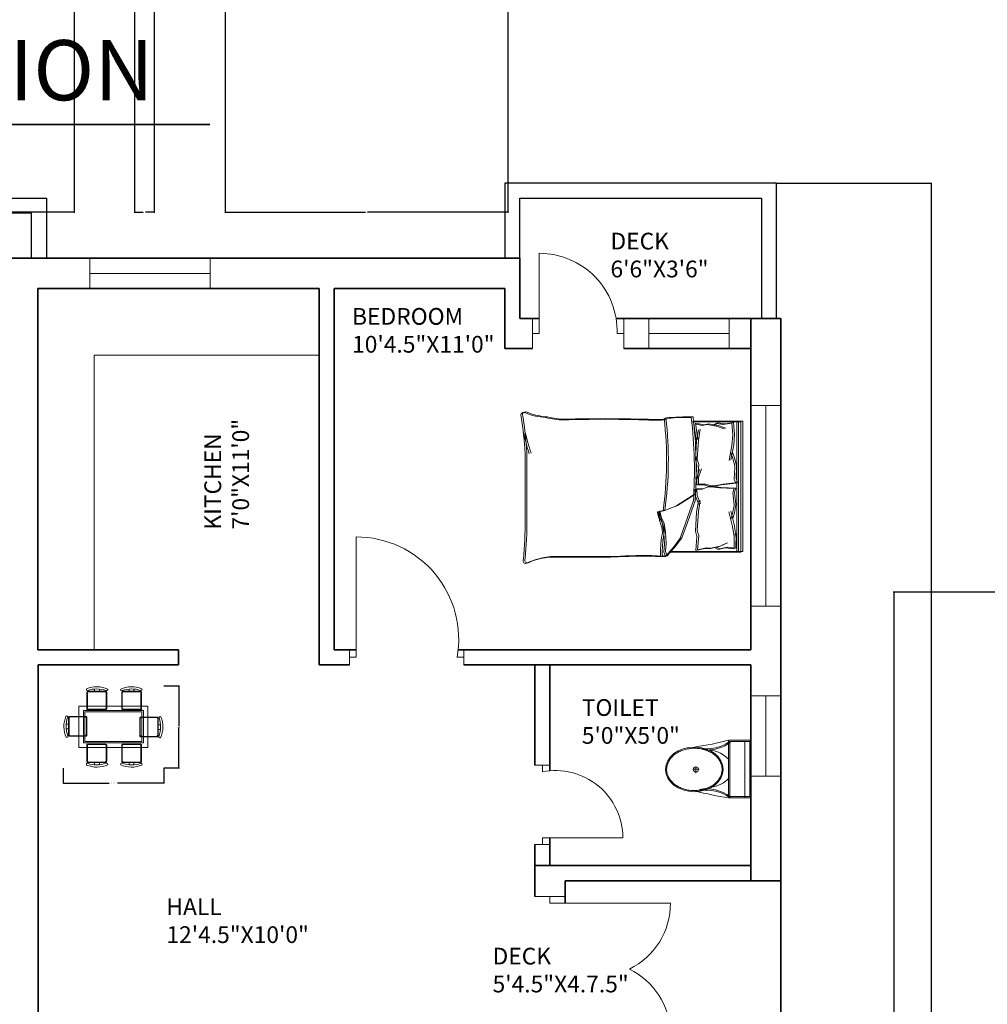
# Model space of a CAD drawing. Units: inches. Extents: x 2250 to 3629, y 982 to 2740.
# Tile 5 of 12: x 2629 to 2918, y 1825 to 2119. Entities that reach past the tile are written whole.
import ezdxf

# ---------------------------------------------------------------- set-up
doc = ezdxf.new("R2010")
doc.units = ezdxf.units.IN
for name, color, linetype, lineweight in [('A-ANNO-DIMS', 2, 'Continuous', 18), ('A-ANNO-TITL', 7, 'Continuous', 35), ('A-AREA-IDEN', 7, 'Continuous', 18), ('A-DOOR', 3, 'Continuous', 18), ('A-FLOR-DECK', 7, 'Continuous', 25), ('A-FLOR-FIXT', 9, 'Continuous', 18), ('A-FURN', 8, 'Continuous', 13), ('A-GLAZ', 4, 'Continuous', 18), ('A-WALL', 7, 'Continuous', 35)]:
    doc.layers.add(name, color=color, linetype=linetype, lineweight=lineweight)
doc.styles.get("Standard").update_dxf_attribs({"font": 'arial.ttf'})
doc.dimstyles.get("Standard").update_dxf_attribs({"dimtxt": 0.18, "dimasz": 0.18, "dimexe": 0.18, "dimexo": 0.0625, "dimgap": 0.09, "dimtad": 0, "dimtih": 1, "dimtoh": 1, "dimdec": 4, "dimzin": 0, "dimdsep": 46, "dimtxsty": 'Standard', "dimcen": 0.09, "dimadec": 0, "dimazin": 0, "dimtfac": 1, "dimtdec": 4, "dimtofl": 0, "dimtmove": 0, "dimatfit": 3, "dimfxl": 1, "dimtolj": 1, "dimtzin": 0, "dimarcsym": 0})

# ---------------------------------------------------------------- blocks, each defined once
blk = doc.blocks.new('A$C31115884')
for p, q in [((283.1, 497.7), (223.4, 497.7)), ((257.5, 466.4), (257.5, 523.2)), ((0, 200), (0, 0)), ((520, 200), (0, 200)), ((10, 190), (10, 10)), ((510, 190), (10, 190)), ((510, 10), (510, 190)), ((520, 0), (520, 200)), ((510, 54.5), (0, 54.5)), ((10, 10), (510, 10)), ((0, 0), (520, 0))]:
    blk.add_line(p, q)
blk.add_circle((255.6, 496.4), 23.6)
for centre, radius, start, end in [((2777.7, -204.6), 2807, 165.4549, 171.71327), ((-294.5, 403.3), 364.7, 324.20913, 9.34987), ((-294.5, 403.3), 374.7, 324.20913, 9.34987), ((805.8, 403.3), 364.7, 170.65013, 215.79087), ((3237, 905), 2807, 188.28673, 194.5451), ((139.5, 406.2), 293.5, 315.84364, 2.65635), ((805.8, 403.3), 374.7, 179.20365, 215.79087), ((383.6, 406.2), 293.5, 190.27735, 224.15636)]:
    blk.add_arc(centre, radius, start, end)
blk.add_ellipse((256.2, 509.9), major_axis=(0, -260.7), ratio=0.772727)
blk.add_open_spline([(256.2, 259.2), (263.1, 259.2), (270, 259.7), (287.8, 262.3), (298.7, 265.1), (319.9, 273.1), (330.2, 278.4), (350.1, 291.1), (359.7, 298.7), (377.7, 315.9), (386.2, 325.5), (401.7, 346.6), (408.8, 358.1), (421.3, 382.5), (426.8, 395.5), (435.9, 422.4), (439.5, 436.4), (444.8, 465.1), (446.5, 479.7), (447.9, 509.2), (447.6, 524), (445, 553.3), (442.7, 567.8), (436.3, 596), (432.1, 609.7), (421.9, 636), (416, 648.6), (402.5, 672.1), (395, 683), (378.6, 703), (369.8, 712.1), (351.1, 728), (341.3, 734.8), (320.9, 746.2), (310.4, 750.7), (288.9, 757.3), (278, 759.4), (256, 761), (245, 760.6), (223.1, 757.2), (212.3, 754.3), (191.1, 746.1), (180.8, 740.7), (160.9, 727.8), (151.4, 720.1), (133.5, 702.7), (125.1, 693), (109.6, 671.7), (102.6, 660.2), (90.2, 635.7), (84.9, 622.7), (76, 595.6), (72.4, 581.6), (67.2, 552.9), (65.6, 538.2), (64.4, 508.8), (64.8, 494), (67.5, 464.7), (69.9, 450.2), (76.6, 422), (80.8, 408.3), (91.1, 382.2), (97.2, 369.7), (110.8, 346.3), (118.4, 335.4), (134.8, 315.6), (143.7, 306.7), (162.4, 290.9), (172.3, 284.2), (192.8, 273), (203.3, 268.6), (224.8, 262.2), (235.8, 260.2), (249.9, 259.3), (253, 259.2), (256.2, 259.2)], degree=3, knots=[0, 0, 0, 0, 0.110105, 0.110105, 0.285049, 0.285049, 0.459994, 0.459994, 0.634938, 0.634938, 0.809882, 0.809882, 0.984827, 0.984827, 1.159771, 1.159771, 1.334715, 1.334715, 1.50966, 1.50966, 1.684604, 1.684604, 1.859549, 1.859549, 2.034493, 2.034493, 2.209437, 2.209437, 2.384382, 2.384382, 2.559326, 2.559326, 2.73427, 2.73427, 2.909215, 2.909215, 3.084159, 3.084159, 3.259103, 3.259103, 3.434048, 3.434048, 3.608992, 3.608992, 3.783936, 3.783936, 3.958881, 3.958881, 4.133825, 4.133825, 4.30877, 4.30877, 4.483714, 4.483714, 4.658658, 4.658658, 4.833603, 4.833603, 5.008547, 5.008547, 5.183491, 5.183491, 5.358436, 5.358436, 5.53338, 5.53338, 5.708324, 5.708324, 5.883269, 5.883269, 6.058213, 6.058213, 6.233158, 6.233158, 6.283185, 6.283185, 6.283185, 6.283185])
blk = doc.blocks.new('DR-36-BED-NE')
for p, q in [((2, 2.25), (2, 38.25)), ((0, 4.5), (0, 0)), ((34.14, 4.5), (34.14, 0)), ((0, 0), (0, 2.25)), ((0, 2.25), (2, 2.25)), ((34.14, 2.25), (32.14, 2.25)), ((34.14, 0), (34.14, 2.25))]:
    blk.add_line(p, q)
blk.add_arc((2, 7.63), 30.62, 349.8775, 90)
blk = doc.blocks.new('DR-24-DECK-NE')
for p, q in [((2, 4.5), (2, 28.5)), ((0, 9), (0, 0)), ((27.25, 9), (27.25, 0)), ((0, 0), (0, 4.5)), ((0, 4.5), (2, 4.5)), ((27.25, 4.5), (25.25, 4.5)), ((27.25, 0), (27.25, 4.5))]:
    blk.add_line(p, q)
blk.add_arc((2, 5.23), 23.27, 358.191, 90)
blk = doc.blocks.new('DR-24-BATH-NE')
for p, q in [((0, 23.65), (4.5, 23.65)), ((4.5, 23.65), (2.25, 23.65)), ((2.25, 23.65), (2.25, 21.65)), ((4.5, 0), (0, 0)), ((0, 0), (0, 0)), ((0, 0), (2.25, 0)), ((2.25, 0), (2.25, 2)), ((2.25, 2), (26.25, 2))]:
    blk.add_line(p, q)
blk.add_arc((6.2, 2), 20.05, 0, 101.3787)
blk = doc.blocks.new('DR-72-DECK-EAST-N')
for p, q in [((9, 42.6), (0, 42.6)), ((0, 42.6), (4.5, 42.6)), ((4.5, 42.6), (4.5, 40.6)), ((4.5, 40.6), (40.5, 40.6)), ((9, 0), (0, 0)), ((0, 0), (4.5, 0)), ((4.5, 0), (4.5, 2)), ((4.5, 2), (40.5, 2))]:
    blk.add_line(p, q)
for centre, radius, start, end in [((18.63, 40.6), 21.87, 295.9981, 0), ((18.59, 1.24), 21.93, 1.9829, 63.9515)]:
    blk.add_arc(centre, radius, start, end)
blk = doc.blocks.new('WIN-24-DECK-NE')
for p, q in [((0, 4.5), (0, 9)), ((0, 9), (0, 0)), ((24, 0), (24, 9)), ((24, 9), (24, 4.5)), ((24, 4.5), (0, 4.5))]:
    blk.add_line(p, q)
blk = doc.blocks.new('WIN-60-BED-NE')
for p, q in [((0, 60), (9, 60)), ((9, 60), (4.5, 60)), ((4.5, 60), (4.5, 12)), ((4.5, 12), (4.5, 0)), ((4.5, 0), (0, 0)), ((0, 0), (9, 0))]:
    blk.add_line(p, q)
blk = doc.blocks.new('WIN-36-KITCHEN-NE')
for p, q in [((0, 9), (0, 0)), ((0, 0), (0, 9)), ((0, 9), (0, 4.5)), ((36, 4.5), (36, 9)), ((36, 9), (36, 0)), ((0, 4.5), (36, 4.5))]:
    blk.add_line(p, q)
blk = doc.blocks.new('WIN-24-BATH-NW')
for p, q in [((9, 24), (0, 24)), ((0, 24), (4.5, 24)), ((4.5, 24), (4.5, 0)), ((9, 0), (0, 0)), ((4.5, 0), (9, 0))]:
    blk.add_line(p, q)
blk = doc.blocks.new('BED-WITH-PILLOWS')
for p, q in [((2.83, 51.56), (2.83, 66.3)), ((2.83, 66.3), (41.74, 66.3)), ((2.83, 65.05), (41.74, 65.05)), ((3.02, 51.04), (3.02, 65.78)), ((3.02, 65.78), (41.92, 65.78)), ((19.98, 64.31), (21.15, 64.78)), ((21.15, 64.78), (21.62, 60.43)), ((41.74, 66.3), (41.74, 44.64)), ((41.92, 65.78), (41.92, 44.12)), ((3.02, 64.53), (41.92, 64.53)), ((3.17, 63.59), (6.66, 63.85)), ((3.17, 63.6), (3.64, 61.01)), ((3.36, 63.06), (6.85, 63.33)), ((3.36, 63.08), (3.83, 60.49)), ((6.66, 63.85), (6.75, 63.84)), ((6.75, 63.84), (9.86, 63.6)), ((6.85, 63.33), (6.93, 63.32)), ((6.93, 63.32), (10.04, 63.08)), ((9.86, 63.6), (14.33, 62.78)), ((10.04, 63.08), (14.52, 62.26)), ((12.09, 63.25), (13.74, 63.84)), ((12.28, 62.73), (13.93, 63.32)), ((13.74, 63.84), (16.09, 64.43)), ((13.93, 63.32), (16.28, 63.91)), ((16.09, 64.43), (16.36, 64.43)), ((16.28, 63.91), (16.54, 63.91)), ((16.36, 64.43), (19.98, 64.31)), ((16.54, 63.91), (20.16, 63.79)), ((20.16, 63.79), (21.34, 64.26)), ((21.34, 64.26), (21.81, 59.9)), ((22.78, 64.27), (22.58, 59.9)), ((22.96, 63.75), (22.76, 59.38)), ((23.98, 63.88), (22.78, 64.27)), ((24.17, 63.36), (22.96, 63.75)), ((27.59, 64.22), (23.98, 63.88)), ((27.77, 63.7), (24.17, 63.36)), ((27.85, 64.24), (27.59, 64.22)), ((28.03, 63.72), (27.77, 63.7)), ((30.23, 63.8), (27.85, 64.24)), ((30.42, 63.28), (28.03, 63.72)), ((34.12, 63.8), (29.71, 62.7)), ((34.31, 63.28), (29.9, 62.18)), ((31.91, 63.31), (30.23, 63.8)), ((32.1, 62.79), (30.42, 63.28)), ((37.22, 64.23), (34.12, 63.8)), ((37.4, 63.71), (34.31, 63.28)), ((40.8, 64.22), (36.4, 64.3)), ((36.4, 64.3), (37.22, 64.23)), ((40.98, 63.7), (36.58, 63.78)), ((36.58, 63.78), (37.4, 63.71)), ((40.8, 64.22), (40.49, 61.61)), ((40.98, 63.7), (40.67, 61.09)), ((3.64, 61.01), (3.29, 58.89)), ((3.29, 58.89), (3.76, 58.07)), ((3.83, 60.49), (3.47, 58.37)), ((3.64, 56.07), (4.11, 59.01)), ((4.11, 59.01), (4.94, 61.25)), ((4.3, 58.49), (5.12, 60.73)), ((21.62, 60.43), (22.09, 57.84)), ((21.81, 59.9), (22.28, 57.32)), ((22.58, 59.9), (22.27, 57.28)), ((22.76, 59.38), (22.46, 56.76)), ((40.14, 59.58), (39.18, 61.76)), ((40.33, 59.06), (39.37, 61.24)), ((40.8, 56.67), (40.14, 59.58)), ((40.98, 56.15), (40.33, 59.06)), ((40.49, 61.61), (40.97, 59.51)), ((40.97, 59.51), (40.55, 58.66)), ((40.67, 61.09), (41.16, 58.99)), ((41.16, 58.99), (40.74, 58.14)), ((3.47, 58.37), (3.95, 57.55)), ((3.88, 54.78), (3.64, 56.07)), ((3.83, 55.55), (4.3, 58.49)), ((22.09, 56.78), (21.62, 55.25)), ((22.28, 56.26), (21.81, 54.73)), ((22.09, 57.84), (22.09, 56.78)), ((22.27, 57.28), (22.34, 56.23)), ((22.28, 57.32), (22.28, 56.26)), ((22.34, 56.23), (22.9, 54.73)), ((22.46, 56.76), (22.52, 55.71)), ((40.64, 55.37), (40.8, 56.67)), ((40.83, 54.85), (40.98, 56.15)), ((3.41, 52.19), (3.88, 54.78)), ((3.59, 51.66), (4.06, 54.25)), ((4.06, 54.25), (3.83, 55.55)), ((5.2, 53.58), (8.48, 53.04)), ((5.38, 53.06), (8.66, 52.52)), ((8.48, 53.04), (7.56, 52.77)), ((8.48, 53.04), (14.18, 52.69)), ((14.18, 52.69), (15.78, 53.14)), ((15.78, 53.14), (19.96, 52.81)), ((19.62, 53.06), (17.06, 53.95)), ((19.81, 52.54), (17.25, 53.43)), ((21.62, 53.06), (19.62, 53.06)), ((21.62, 55.25), (21.62, 53.06)), ((21.81, 54.73), (21.81, 52.54)), ((22.52, 55.71), (23.09, 54.21)), ((22.9, 54.73), (23.04, 52.55)), ((23.09, 54.21), (23.22, 52.03)), ((25.03, 52.68), (27.53, 53.72)), ((25.22, 52.15), (27.72, 53.2)), ((26.51, 53.58), (29.79, 53.04)), ((26.7, 53.06), (29.98, 52.52)), ((29.79, 53.04), (35.5, 52.69)), ((35.5, 52.69), (37.1, 53.14)), ((37.1, 53.14), (41.27, 52.81)), ((41.27, 52.81), (40.64, 55.37)), ((41.46, 52.29), (40.83, 54.85)), ((7.56, 52.77), (3.41, 52.19)), ((7.74, 52.25), (3.59, 51.66)), ((8.66, 52.52), (7.74, 52.25)), ((8.66, 52.52), (14.37, 52.17)), ((14.37, 52.17), (15.97, 52.62)), ((15.97, 52.62), (20.14, 52.29)), ((21.81, 52.54), (19.81, 52.54)), ((23.04, 52.55), (25.03, 52.68)), ((23.22, 52.03), (25.22, 52.15)), ((24.63, 52.15), (28.05, 46.86)), ((24.82, 51.63), (28.23, 46.34)), ((33.09, 49.76), (26.3, 52.15)), ((33.27, 49.24), (26.49, 51.63)), ((29.98, 52.52), (35.69, 52.17)), ((35.69, 52.17), (37.28, 52.62)), ((37.28, 52.62), (41.46, 52.29)), ((37.63, 48.12), (33.09, 49.76)), ((37.81, 47.6), (33.27, 49.24)), ((40.02, 46.36), (37.63, 48.12)), ((40.21, 45.84), (37.81, 47.6)), ((28.05, 46.86), (29.43, 43.21)), ((28.23, 46.34), (29.62, 42.69)), ((43.04, 43.71), (40.02, 46.36)), ((43.23, 43.19), (40.21, 45.84)), ((29.43, 43.21), (29.68, 41.57)), ((29.62, 42.69), (29.87, 41.05)), ((29.68, 41.57), (31.7, 42.08)), ((29.87, 41.05), (31.89, 41.56)), ((31.7, 42.08), (33.34, 42.83)), ((31.89, 41.56), (33.53, 42.31)), ((33.34, 42.83), (36.11, 43.21)), ((33.53, 42.31), (36.3, 42.69)), ((36.11, 43.21), (39.27, 43.46)), ((36.3, 42.69), (39.45, 42.94)), ((39.27, 43.46), (41.79, 43.21)), ((39.45, 42.94), (41.97, 42.69)), ((41.79, 43.21), (43.04, 43.71)), ((41.97, 42.69), (43.23, 43.19)), ((43.1, 42.29), (43.04, 43.71, 3.15)), ((43.29, 41.77), (43.23, 43.19, 3.15)), ((12.26, 1.79), (32.3, 1.79)), ((12.45, 1.27), (32.49, 1.27))]:
    blk.add_line(p, q)
for centre, radius, start, end in [((69.33, 49.94), 67.82, 178.7218, 185.604), ((17.39, -81.91), 134.3, 86.0865, 96.7821), ((69.52, 49.42), 67.82, 178.7218, 185.604), ((17.57, -82.43), 134.3, 86.0865, 96.7821), ((14.46, -60.96), 105.04, 81.7845, 96.9006), ((14.64, -61.48), 105.04, 81.7845, 96.9006), ((-136.21, 40.92), 138.49, 358.4762, 1.0082), ((-136.02, 40.4), 138.49, 358.4762, 1.0082), ((29.83, 41.52), 0.15, 160.2464, 271.1377), ((25.36, 65.1), 24.14, 280.6617, 289.8806), ((25.55, 64.58), 24.14, 280.6617, 289.8806), ((35.61, 37.76), 5.07, 78.6608, 113.7384), ((35.8, 37.23), 5.07, 78.6608, 113.7384), ((41.79, 71.72), 29.46, 259.8763, 272.5657), ((41.97, 71.2), 29.46, 259.8763, 272.5657), ((148.38, 36.74), 105.43, 176.9791, 183.8365), ((148.57, 36.22), 105.43, 176.9791, 183.8365), ((30.01, 41), 0.15, 160.2464, 271.1377), ((394.7, 25.1), 392.65, 178.2277, 181.7185), ((394.88, 24.58), 392.65, 178.2277, 181.7185), ((-3670.6, 11.09), 3713.84, 0.00217, 0.28689), ((-3670.41, 10.57), 3713.84, 0.00217, 0.28689), ((-21.9, 13.78), 24.13, 346.0648, 358.9113), ((-21.71, 13.26), 24.13, 346.0648, 358.9113), ((62, 10.4), 18.78, 177.4714, 206.4681), ((62.19, 9.88), 18.78, 177.4714, 206.4681), ((-17.63, 9.09), 19.18, 337.9751, 356.652), ((-17.45, 8.57), 19.18, 337.9751, 356.652), ((-14.02, 85.61), 86.67, 283.3832, 287.7053), ((0.89, 1.4), 0.887, 146.1736, 293.4781), ((1.07, 0.88), 0.887, 146.1736, 293.4781), ((17.44, -97.2), 99.12, 92.9958, 99.4091), ((17.63, -97.72), 99.12, 92.9958, 99.4091), ((-13.83, 85.09), 86.67, 283.3832, 287.7053), ((33.5, -106.51), 108.31, 84.4998, 90.6351), ((33.69, -107.03), 108.31, 84.4998, 90.6351), ((44.3, 2.09), 0.897, 242.6588, 356.02), ((44.48, 1.57), 0.897, 242.6588, 356.02)]:
    blk.add_arc(centre, radius, start, end)
blk = doc.blocks.new('DINING-SET-6')
for points in [[(7.06, 22.9, -0.175809), (12.68, 22.86, 0.578392), (13.1, 23.32, 0.214524), (6.77, 23.41, 0.552014), (7.06, 22.9, -0.065079)], [(17.4, 22.86, -0.578392), (16.98, 23.32, -0.214524), (23.31, 23.41, -0.552014), (23.02, 22.9, 0.175809), (17.4, 22.86)], [(12.44, 22.67), (7.23, 22.67, 0.414214), (6.86, 22.31), (6.86, 17.52, 0.414214), (7.23, 17.15), (12.44, 17.15, 0.414214), (12.8, 17.52), (12.8, 22.31, 0.414214), (12.44, 22.67)], [(10.61, 22.67), (10.61, 23.33, -0.064759)], [(22.85, 22.67, -0.414214), (23.22, 22.31), (23.22, 17.52, -0.414214), (22.85, 17.15), (17.64, 17.15, -0.414214), (17.28, 17.52), (17.28, 22.31, -0.414214), (17.64, 22.67), (22.85, 22.67)], [(19.47, 22.67), (19.47, 23.33, 0.064759)], [(1.19, 9.34, -0.578392), (0.72, 8.92, -0.214524), (0.64, 15.25, -0.552014), (1.15, 14.96, 0.175809), (1.19, 9.34)], [(1.37, 14.79, -0.414214), (1.74, 15.16), (6.53, 15.16, -0.414214), (6.89, 14.79), (6.89, 9.58, -0.414214), (6.53, 9.22), (1.74, 9.22, -0.414214), (1.37, 9.58), (1.37, 14.79)], [(28.21, 14.61, 0.414214), (27.85, 14.98), (23.05, 14.98, 0.414214), (22.69, 14.61), (22.69, 9.4, 0.414214), (23.05, 9.04), (27.85, 9.04, 0.414214), (28.21, 9.4), (28.21, 14.61)], [(28.44, 14.78, -0.175809), (28.39, 9.16, 0.578392), (28.86, 8.74, 0.214524), (28.95, 15.08, 0.552014), (28.44, 14.78, -0.065079)], [(1.37, 11.41), (0.71, 11.41, 0.064759)], [(28.21, 11.23), (28.87, 11.23, -0.064759)], [(12.44, 1.37), (7.23, 1.37, -0.414214), (6.86, 1.74), (6.86, 6.53, -0.414214), (7.23, 6.89), (12.44, 6.89, -0.414214), (12.8, 6.53), (12.8, 1.74, -0.414214), (12.44, 1.37)], [(22.85, 1.37, 0.414214), (23.22, 1.74), (23.22, 6.53, 0.414214), (22.85, 6.89), (17.64, 6.89, 0.414214), (17.28, 6.53), (17.28, 1.74, 0.414214), (17.64, 1.37), (22.85, 1.37)], [(12.68, 1.19, -0.578392), (13.1, 0.72, -0.214524), (6.77, 0.64, -0.552014), (7.06, 1.15, 0.175809), (12.68, 1.19)], [(10.61, 1.37), (10.61, 0.71, 0.064759)], [(23.02, 1.15, -0.175809), (17.4, 1.19, 0.578392), (16.98, 0.72, 0.214524), (23.31, 0.64, 0.552014), (23.02, 1.15, -0.065079)], [(19.47, 1.37), (19.47, 0.71, -0.064759)]]:
    blk.add_lwpolyline(points, format="xyb")
for points in [[(7.23, 22.51), (12.27, 22.51, -0.414214), (12.64, 22.15), (12.64, 17.68, -0.414214), (12.27, 17.32), (7.23, 17.32, -0.512069), (7.03, 17.68), (7.03, 22.15, -0.512069)], [(22.85, 22.51), (17.81, 22.51, 0.414214), (17.44, 22.15), (17.44, 17.68, 0.414214), (17.81, 17.32), (22.85, 17.32, 0.512069), (23.05, 17.68), (23.05, 22.15, 0.512069)], [(1.54, 14.79), (1.54, 9.75, 0.414214), (1.9, 9.38), (6.37, 9.38, 0.414214), (6.73, 9.75), (6.73, 14.79, 0.512069), (6.37, 14.99), (1.9, 14.99, 0.512069)], [(28.05, 14.61), (28.05, 9.57, -0.414214), (27.68, 9.2), (23.22, 9.2, -0.414214), (22.85, 9.57), (22.85, 14.61, -0.512069), (23.22, 14.81), (27.68, 14.81, -0.512069)], [(7.23, 1.54), (12.27, 1.54, 0.414214), (12.64, 1.9), (12.64, 6.36, 0.414214), (12.27, 6.73), (7.23, 6.73, 0.512069), (7.03, 6.36), (7.03, 1.9, 0.512069)], [(22.85, 1.54), (17.81, 1.54, -0.414214), (17.44, 1.9), (17.44, 6.36, -0.414214), (17.81, 6.73), (22.85, 6.73, -0.512069), (23.05, 6.36), (23.05, 1.9, -0.512069)]]:
    blk.add_lwpolyline(points, format="xyb", close=True)
for points in [[(9.15, 23.35), (9.15, 22.67)], [(20.93, 23.35), (20.93, 22.67)], [(0.7, 12.87), (1.37, 12.87)], [(28.88, 12.69), (28.21, 12.69)], [(9.15, 0.7), (9.15, 1.37)], [(20.93, 0.7), (20.93, 1.37)]]:
    blk.add_lwpolyline(points)
for points in [[(4.51, 18.27), (25.12, 18.27), (25.12, 5.91), (4.51, 5.91)], [(5.89, 16.9), (23.75, 16.9), (23.75, 7.28), (5.89, 7.28)], [(6.3, 16.49), (23.34, 16.49), (23.34, 7.69), (6.3, 7.69)]]:
    blk.add_lwpolyline(points, close=True)
blk = doc.blocks.new('*D61')
at = {"layer": 'A-ANNO-DIMS', "color": 0, "lineweight": -2, "transparency": 16777216}
for p, q in [((2642.11, 1895.36), (2642.11, 1890.73)), ((2672.18, 1895.36), (2672.18, 1890.73)), ((2642.29, 1890.91), (2655.86, 1890.91)), ((2672, 1890.91), (2658.42, 1890.91))]:
    blk.add_line(p, q, dxfattribs=at)
at = {"layer": 'A-ANNO-DIMS', "color": 0, "transparency": 16777216}
for points in [[(2642.29, 1890.94), (2642.29, 1890.88), (2642.11, 1890.91)], [(2672, 1890.94), (2672, 1890.88), (2672.18, 1890.91)]]:
    blk.add_solid(points, dxfattribs=at)
at = {"layer": 'Defpoints', "color": 0, "transparency": 16777216}
for p in [(2642.11, 1895.42), (2672.18, 1895.42), (2672.18, 1890.91)]:
    blk.add_point(p, dxfattribs=at)
at = {"layer": 'A-ANNO-DIMS', "color": 0, "transparency": 16777216, "insert": (2657.14, 1890.91), "char_height": 0.18, "attachment_point": 5}
blk.add_mtext('\\A1;DINING SET 30 TYP.', dxfattribs=at)
blk = doc.blocks.new('*D62')
at = {"layer": 'A-ANNO-DIMS', "color": 0, "lineweight": -2, "transparency": 16777216}
for p, q in [((2672.24, 1919.95), (2676.87, 1919.95)), ((2676.69, 1919.77), (2676.69, 1907.87)), ((2676.69, 1895.6), (2676.69, 1907.5)), ((2672.24, 1895.42), (2676.87, 1895.42))]:
    blk.add_line(p, q, dxfattribs=at)
at = {"layer": 'A-ANNO-DIMS', "color": 0, "transparency": 16777216}
for points in [[(2676.66, 1919.77), (2676.72, 1919.77), (2676.69, 1919.95)], [(2676.66, 1895.6), (2676.72, 1895.6), (2676.69, 1895.42)]]:
    blk.add_solid(points, dxfattribs=at)
at = {"layer": 'Defpoints', "color": 0, "transparency": 16777216}
for p in [(2672.18, 1919.95), (2676.69, 1919.95), (2672.18, 1895.42)]:
    blk.add_point(p, dxfattribs=at)
at = {"layer": 'A-ANNO-DIMS', "color": 0, "transparency": 16777216, "insert": (2676.69, 1907.69), "char_height": 0.18, "attachment_point": 5}
blk.add_mtext('\\A1;25 TYP.', dxfattribs=at)
blk = doc.blocks.new('*D170')
at = {"layer": 'A-ANNO-DIMS', "color": 0, "lineweight": -2, "transparency": 16777216}
for p, q in [((2855.4, 2070.24), (2901.69, 2070.24)), ((2901.51, 2070.06), (2901.51, 1664.67)), ((2901.51, 1258.92), (2901.51, 1664.3)), ((2481.67, 1258.74), (2901.69, 1258.74))]:
    blk.add_line(p, q, dxfattribs=at)
at = {"layer": 'A-ANNO-DIMS', "color": 0, "transparency": 16777216}
for points in [[(2901.48, 2070.06), (2901.54, 2070.06), (2901.51, 2070.24)], [(2901.48, 1258.92), (2901.54, 1258.92), (2901.51, 1258.74)]]:
    blk.add_solid(points, dxfattribs=at)
at = {"layer": 'Defpoints', "color": 0, "transparency": 16777216}
for p in [(2855.34, 2070.24), (2901.51, 2070.24), (2481.61, 1258.74)]:
    blk.add_point(p, dxfattribs=at)
at = {"layer": 'A-ANNO-DIMS', "color": 0, "transparency": 16777216, "insert": (2901.51, 1664.49), "char_height": 0.18, "attachment_point": 5}
blk.add_mtext('\\A1;811.5', dxfattribs=at)
blk = doc.blocks.new('*D173')
at = {"layer": 'A-ANNO-DIMS', "color": 0, "lineweight": -2, "transparency": 16777216}
for p, q in [((2932.01, 1947.92), (2890.14, 1947.92)), ((2890.32, 1947.74), (2890.32, 1603.51)), ((2890.32, 1258.92), (2890.32, 1603.15)), ((2981.16, 1258.74), (2890.14, 1258.74))]:
    blk.add_line(p, q, dxfattribs=at)
at = {"layer": 'A-ANNO-DIMS', "color": 0, "transparency": 16777216}
for points in [[(2890.29, 1947.74), (2890.35, 1947.74), (2890.32, 1947.92)], [(2890.29, 1258.92), (2890.35, 1258.92), (2890.32, 1258.74)]]:
    blk.add_solid(points, dxfattribs=at)
at = {"layer": 'Defpoints', "color": 0, "transparency": 16777216}
for p in [(2932.07, 1947.92), (2890.32, 1258.74), (2981.23, 1258.74)]:
    blk.add_point(p, dxfattribs=at)
at = {"layer": 'A-ANNO-DIMS', "color": 0, "transparency": 16777216, "insert": (2890.32, 1603.33), "char_height": 0.18, "attachment_point": 5}
blk.add_mtext('\\A1;689.2', dxfattribs=at)
blk = doc.blocks.new('*D184')
at = {"layer": 'A-ANNO-DIMS', "color": 0, "lineweight": -2, "transparency": 16777216}
for p, q in [((2645.41, 2191.68), (2645.41, 2061.34)), ((2597.69, 2173.64), (2597.69, 2061.34)), ((2597.87, 2061.52), (2621.08, 2061.52)), ((2645.23, 2061.52), (2622.02, 2061.52))]:
    blk.add_line(p, q, dxfattribs=at)
at = {"layer": 'A-ANNO-DIMS', "color": 0, "transparency": 16777216}
for points in [[(2597.87, 2061.55), (2597.87, 2061.49), (2597.69, 2061.52)], [(2645.23, 2061.55), (2645.23, 2061.49), (2645.41, 2061.52)]]:
    blk.add_solid(points, dxfattribs=at)
at = {"layer": 'Defpoints', "color": 0, "transparency": 16777216}
for p in [(2645.41, 2191.74), (2597.69, 2173.7), (2645.41, 2061.52)]:
    blk.add_point(p, dxfattribs=at)
at = {"layer": 'A-ANNO-DIMS', "color": 0, "transparency": 16777216, "insert": (2621.55, 2061.52), "char_height": 0.18, "attachment_point": 5}
blk.add_mtext('\\A1;47.725', dxfattribs=at)
blk = doc.blocks.new('*D185')
at = {"layer": 'A-ANNO-DIMS', "color": 0, "lineweight": -2, "transparency": 16777216}
for p, q in [((2663.46, 2191.6), (2663.46, 2061.34)), ((2669.31, 2191.64), (2669.31, 2061.34)), ((2663.64, 2061.52), (2666.06, 2061.52)), ((2669.13, 2061.52), (2666.71, 2061.52))]:
    blk.add_line(p, q, dxfattribs=at)
at = {"layer": 'A-ANNO-DIMS', "color": 0, "transparency": 16777216}
for points in [[(2663.64, 2061.55), (2663.64, 2061.49), (2663.46, 2061.52)], [(2669.13, 2061.55), (2669.13, 2061.49), (2669.31, 2061.52)]]:
    blk.add_solid(points, dxfattribs=at)
at = {"layer": 'Defpoints', "color": 0, "transparency": 16777216}
for p in [(2663.46, 2191.66), (2669.31, 2191.7), (2669.31, 2061.52)]:
    blk.add_point(p, dxfattribs=at)
at = {"layer": 'A-ANNO-DIMS', "color": 0, "transparency": 16777216, "insert": (2666.38, 2061.52), "char_height": 0.18, "attachment_point": 5}
blk.add_mtext('\\A1;5.85', dxfattribs=at)
blk = doc.blocks.new('*D186')
at = {"layer": 'A-ANNO-DIMS', "color": 0, "lineweight": -2, "transparency": 16777216}
for p, q in [((2690.54, 2191.64), (2690.54, 2061.34)), ((2775.05, 2173.64), (2775.05, 2061.34)), ((2690.72, 2061.52), (2732.47, 2061.52)), ((2774.87, 2061.52), (2733.12, 2061.52))]:
    blk.add_line(p, q, dxfattribs=at)
at = {"layer": 'A-ANNO-DIMS', "color": 0, "transparency": 16777216}
for points in [[(2690.72, 2061.55), (2690.72, 2061.49), (2690.54, 2061.52)], [(2774.87, 2061.55), (2774.87, 2061.49), (2775.05, 2061.52)]]:
    blk.add_solid(points, dxfattribs=at)
at = {"layer": 'Defpoints', "color": 0, "transparency": 16777216}
for p in [(2690.54, 2191.7), (2775.05, 2173.7), (2775.05, 2061.52)]:
    blk.add_point(p, dxfattribs=at)
at = {"layer": 'A-ANNO-DIMS', "color": 0, "transparency": 16777216, "insert": (2732.8, 2061.52), "char_height": 0.18, "attachment_point": 5}
blk.add_mtext('\\A1;84.5', dxfattribs=at)

msp = doc.modelspace()

# ---------------------------------------------------------------- linework, layer by layer
at = {"layer": 'A-ANNO-TITL'}
msp.add_line((2533.1975, 2087.7229), (2686.0181, 2087.7229), dxfattribs=at)
at = {"layer": 'A-FLOR-DECK'}
for p, q in [((2855.3384, 2070.2354), (2774.1072, 2070.2354)), ((2774.1072, 2070.2354), (2774.1072, 2047.7354)), ((2855.3384, 2065.7354), (2855.3384, 2070.2354)), ((2562.1345, 2065.7354), (2637.208, 2065.7354)), ((2637.208, 2065.7354), (2637.208, 2047.7354)), ((2778.6072, 2047.7354), (2778.6072, 2065.7354)), ((2778.6072, 2065.7354), (2850.8384, 2065.7354)), ((2850.8384, 2065.7354), (2850.8384, 2029.7354)), ((2855.3384, 2029.7354), (2855.3384, 2065.7354)), ((2632.708, 2061.2354), (2566.6345, 2061.2354)), ((2632.708, 2047.7354), (2632.708, 2061.2354)), ((2637.208, 2047.7354), (2632.708, 2047.7354))]:
    msp.add_line(p, q, dxfattribs=at)
at = {"layer": 'A-FLOR-FIXT'}
for p, q in [((2651.3954, 1930.7354), (2651.3954, 2018.7457)), ((2651.3954, 2018.7457), (2718.6072, 2018.7457))]:
    msp.add_line(p, q, dxfattribs=at)
at = {"layer": 'A-WALL'}
for p, q in [((2625.6072, 2047.7354), (2778.6072, 2047.7354)), ((2778.6072, 2047.7354), (2778.6072, 2029.7354)), ((2634.6072, 2038.7354), (2634.6072, 1930.7354)), ((2634.6072, 2038.7354), (2718.6072, 2038.7354)), ((2718.6072, 2038.7354), (2718.6072, 1930.7354)), ((2723.1072, 2038.7354), (2723.1072, 1930.7354)), ((2723.1072, 2038.7354), (2774.1072, 2038.7354)), ((2774.1072, 2020.7354), (2774.1072, 2038.7354)), ((2778.6072, 2029.7354), (2784.402, 2029.7354)), ((2807.3608, 2029.7354), (2847.6072, 2029.7354)), ((2847.6072, 2029.7354), (2847.6072, 1930.7354)), ((2847.6072, 2029.7354), (2847.6072, 2020.7354)), ((2847.6072, 2029.7354), (2856.6072, 2029.7354)), ((2856.6072, 2029.7354), (2856.6072, 1276.7354)), ((2778.6072, 2020.7354), (2774.1072, 2020.7354)), ((2782.402, 2020.7354), (2778.6072, 2020.7354)), ((2847.6072, 2020.7354), (2809.656, 2020.7354)), ((2634.6072, 1930.7354), (2676.6072, 1930.7354)), ((2676.6072, 1930.7354), (2676.6072, 1926.2354)), ((2718.6072, 1930.7354), (2718.6072, 1926.2354)), ((2723.1072, 1930.7354), (2729.7087, 1930.7354)), ((2760.1669, 1930.7354), (2847.6072, 1930.7354)), ((2634.7014, 1926.2354), (2634.7014, 1789.7354)), ((2634.7014, 1926.2354), (2676.6072, 1926.2354)), ((2718.6072, 1926.2354), (2727.7087, 1926.2354)), ((2761.8508, 1926.2354), (2847.6072, 1926.2354)), ((2783.1072, 1896.2354), (2783.1072, 1926.2354)), ((2847.6072, 1926.2354), (2787.6072, 1926.2354)), ((2787.6072, 1926.2354), (2787.6072, 1894.5568)), ((2847.6072, 1926.2354), (2847.6072, 1861.7354)), ((2787.6072, 1874.5842), (2787.6072, 1866.2354)), ((2783.1072, 1866.2354), (2783.1072, 1872.5842)), ((2783.1072, 1866.2354), (2847.6072, 1866.2354)), ((2787.6072, 1866.2354), (2783.1072, 1866.2354)), ((2783.1072, 1866.2354), (2783.1072, 1856.9787)), ((2792.1072, 1861.7354), (2856.6072, 1861.7354)), ((2792.1072, 1854.9787), (2792.1072, 1861.7354))]:
    msp.add_line(p, q, dxfattribs=at)

# ---------------------------------------------------------------- block references
at = {"layer": 'A-DOOR'}
for name, p in [('DR-24-DECK-NE', (2782.402, 2020.735)), ('DR-36-BED-NE', (2727.709, 1926.235)), ('DR-24-BATH-NE', (2783.107, 1872.584)), ('DR-72-DECK-EAST-N', (2783.107, 1814.38))]:
    msp.add_blockref(name, p, dxfattribs=at)
at = {"layer": 'A-FLOR-FIXT', "xscale": 0.0330640103915726, "yscale": 0.0330640103915726, "zscale": 0.0330640103915726, "rotation": 89.99999999999991}
msp.add_blockref('A$C31115884', (2847.6072, 1886.5163), dxfattribs=at)
at = {"layer": 'A-FURN', "rotation": 270}
msp.add_blockref('BED-WITH-PILLOWS', (2778.8948, 2001.8631), dxfattribs=at)
at = {"layer": 'A-FURN'}
msp.add_blockref('DINING-SET-6', (2642.351, 1895.663), dxfattribs=at)
at = {"layer": 'A-GLAZ'}
for name, p in [('WIN-36-KITCHEN-NE', (2650.118, 2038.735)), ('WIN-24-DECK-NE', (2817.153, 2020.735)), ('WIN-60-BED-NE', (2847.607, 1943.78)), ('WIN-24-BATH-NW', (2847.607, 1893.0165))]:
    msp.add_blockref(name, p, dxfattribs=at)

# ---------------------------------------------------------------- texts
at = {"layer": 'A-ANNO-TITL', "insert": (2540.0175, 2112.9477), "char_height": 18, "attachment_point": 1}
msp.add_mtext_dynamic_manual_height_columns('ELEVATION', width=205.216526, gutter_width=12.5, heights=[0], dxfattribs=at)
at = {"layer": 'A-AREA-IDEN', "char_height": 5, "attachment_point": 1}
for s, width, insert in [('DECK\\P6\'6"X3\'6"', 81.726251, (2805.6743, 2055.3736)), ('BEDROOM\\P10\'4.5"X11\'0"', 125.943192, (2728.4706, 2032.8783)), ('TOILET\\P5\'0"X5\'0"', 117.662595, (2797.1133, 1915.9806)), ('HALL\\P12\'4.5"X10\'0"', 122.050361, (2672.9968, 1856.443)), ('DECK\\P5\'4.5"X4.7.5"', 79.279252, (2770.4499, 1841.6872))]:
    msp.add_mtext_dynamic_manual_height_columns(s, width=width, gutter_width=12.5, heights=[0], dxfattribs=dict(at, insert=insert))
at = {"layer": 'A-AREA-IDEN', "insert": (2684.3481, 1966.6619), "char_height": 5, "attachment_point": 1, "rotation": 90}
msp.add_mtext_dynamic_manual_height_columns('KITCHEN\\P7\'0"X11\'0"', width=144.499574, gutter_width=12.5, heights=[0], dxfattribs=at)

# ---------------------------------------------------------------- dimensions: what is measured, and where the dimension line sits
at = {"layer": 'A-ANNO-DIMS'}
for base, p1, p2, override, picture, middle in [((2645.4141, 2061.5229), (2597.6892, 2173.6999), (2645.4141, 2191.7387), {"dimdec": 3, "dimlfac": 1, "dimrnd": 0, "dimzin": 0, "dimdsep": 46, "dimlunit": 2}, '*D184', (2621.5517, 2061.5229)), ((2669.3082, 2061.5229), (2663.4583, 2191.6608), (2669.3082, 2191.6999), {"dimdec": 2, "dimlfac": 1, "dimrnd": 0, "dimzin": 0, "dimdsep": 46, "dimlunit": 2}, '*D185', (2666.3832, 2061.5229)), ((2775.0497, 2061.5229), (2690.5428, 2191.6999), (2775.0497, 2173.6999), {"dimdec": 1, "dimlfac": 1, "dimrnd": 0, "dimzin": 0, "dimdsep": 46, "dimlunit": 2}, '*D186', (2732.7962, 2061.5229))]:
    dim = msp.add_linear_dim(base=base, p1=p1, p2=p2, dimstyle='Standard', override=override, dxfattribs=at)
    dim.commit()
    dim.dimension.update_dxf_attribs({"geometry": picture, "text_midpoint": middle})
for base, p1, p2, picture, middle in [((2901.5072, 2070.2354), (2481.6072, 1258.7354), (2855.3384, 2070.2354), '*D170', (2901.5072, 1664.4854)), ((2890.3241, 1258.7354), (2932.0741, 1947.9231), (2981.2267, 1258.7354), '*D173', (2890.3241, 1603.3293))]:
    dim = msp.add_linear_dim(base=base, p1=p1, p2=p2, angle=90, dimstyle='Standard', override={"dimdec": 1, "dimlfac": 1, "dimrnd": 0, "dimzin": 0, "dimdsep": 46, "dimlunit": 2}, dxfattribs=at)
    dim.commit()
    dim.dimension.update_dxf_attribs({"geometry": picture, "text_midpoint": middle})
dim = msp.add_linear_dim(base=(2676.6859, 1919.9517), p1=(2672.1759, 1895.421), p2=(2672.1759, 1919.9517), angle=90, text='<> TYP.', dimstyle='Standard', override={"dimdec": 0, "dimlfac": 1, "dimrnd": 0, "dimzin": 0, "dimdsep": 46, "dimlunit": 2}, dxfattribs=at)
dim.commit()
dim.dimension.update_dxf_attribs({"geometry": '*D62', "text_midpoint": (2676.6859, 1907.6863)})
dim = msp.add_linear_dim(base=(2672.1759, 1890.911), p1=(2642.1093, 1895.421), p2=(2672.1759, 1895.421), text='DINING SET <> TYP.', dimstyle='Standard', override={"dimdec": 0, "dimlfac": 1, "dimrnd": 0, "dimzin": 0, "dimdsep": 46, "dimlunit": 2}, dxfattribs=at)
dim.commit()
dim.dimension.update_dxf_attribs({"geometry": '*D61', "text_midpoint": (2657.1426, 1890.911)})

doc.saveas('drawing.dxf')
